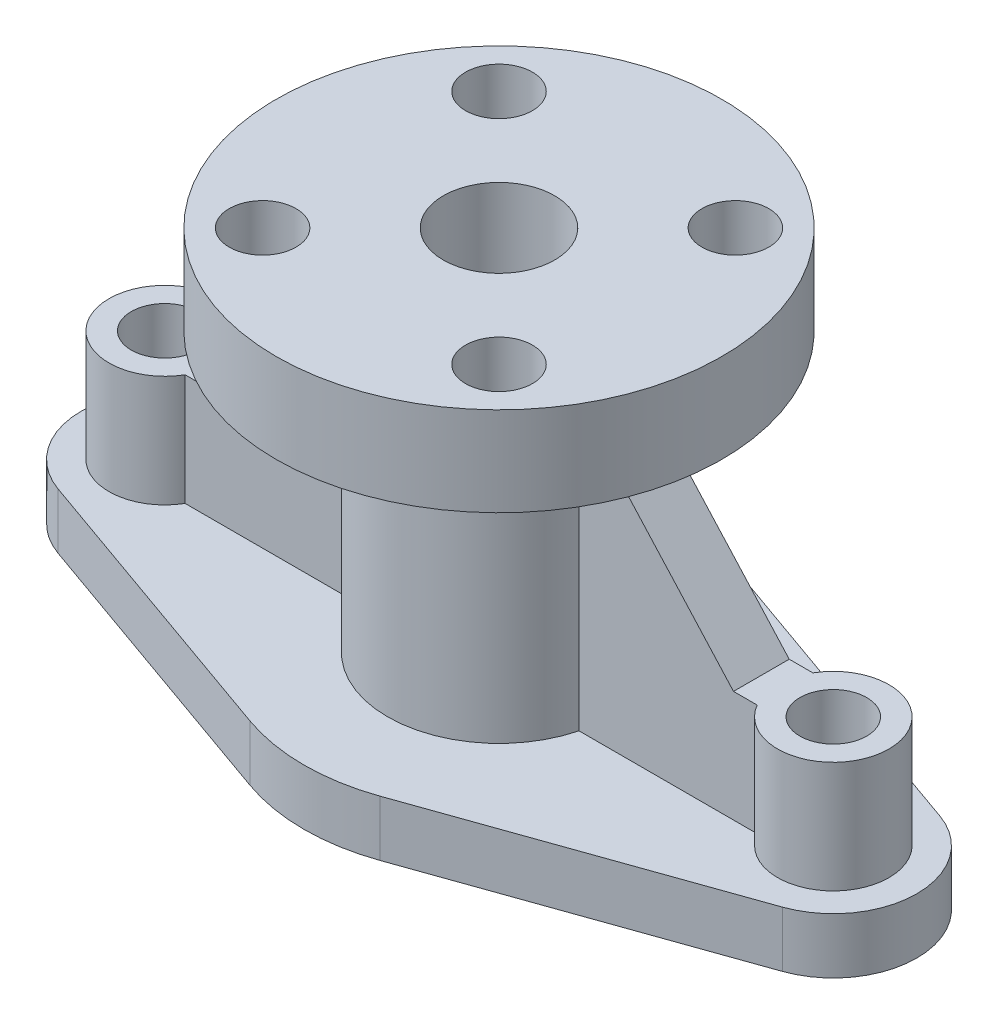
ISO-10303-21;
HEADER;
FILE_DESCRIPTION(('STEP AP214'),'2;1');
FILE_NAME('part.step','',(''),(''),'','','');
FILE_SCHEMA(('AUTOMOTIVE_DESIGN { 1 0 10303 214 1 1 1 1 }'));
ENDSEC;
DATA;
#1=APPLICATION_CONTEXT('core data for automotive mechanical design processes');
#2=APPLICATION_PROTOCOL_DEFINITION('international standard','automotive_design',2000,#1);
#3=PRODUCT_CONTEXT('',#1,'mechanical');
#4=PRODUCT('Part','Part','',(#3));
#5=PRODUCT_RELATED_PRODUCT_CATEGORY('part','',(#4));
#6=PRODUCT_DEFINITION_FORMATION('','',#4);
#7=PRODUCT_DEFINITION_CONTEXT('part definition',#1,'design');
#8=PRODUCT_DEFINITION('design','',#6,#7);
#9=PRODUCT_DEFINITION_SHAPE('','',#8);
#10=(LENGTH_UNIT() NAMED_UNIT(*) SI_UNIT(.MILLI.,.METRE.));
#11=(NAMED_UNIT(*) PLANE_ANGLE_UNIT() SI_UNIT($,.RADIAN.));
#12=(NAMED_UNIT(*) SI_UNIT($,.STERADIAN.) SOLID_ANGLE_UNIT());
#13=UNCERTAINTY_MEASURE_WITH_UNIT(LENGTH_MEASURE(1.E-05),#10,'distance_accuracy_value','');
#14=(GEOMETRIC_REPRESENTATION_CONTEXT(3) GLOBAL_UNCERTAINTY_ASSIGNED_CONTEXT((#13)) GLOBAL_UNIT_ASSIGNED_CONTEXT((#10,
#11,#12)) REPRESENTATION_CONTEXT('',''));
#15=CARTESIAN_POINT('',(0.,0.,0.));
#16=DIRECTION('',(0.,0.,1.));
#17=DIRECTION('',(1.,0.,0.));
#18=AXIS2_PLACEMENT_3D('',#15,#16,#17);
#19=CARTESIAN_POINT('',(0.,10.,0.));
#20=DIRECTION('',(0.,-1.,0.));
#21=DIRECTION('',(0.,0.,-1.));
#22=AXIS2_PLACEMENT_3D('',#19,#20,#21);
#23=CYLINDRICAL_SURFACE('',#22,5.);
#24=CARTESIAN_POINT('',(0.,0.,0.));
#25=DIRECTION('',(0.,1.,0.));
#26=DIRECTION('',(0.,0.,1.));
#27=AXIS2_PLACEMENT_3D('',#24,#25,#26);
#28=CIRCLE('',#27,5.);
#29=CARTESIAN_POINT('',(0.,0.,5.));
#30=VERTEX_POINT('',#29);
#31=EDGE_CURVE('E241',#30,#30,#28,.T.);
#32=ORIENTED_EDGE('',*,*,#31,.F.);
#33=EDGE_LOOP('',(#32));
#34=FACE_BOUND('',#33,.T.);
#35=CARTESIAN_POINT('',(0.,45.,0.));
#36=DIRECTION('',(0.,1.,0.));
#37=DIRECTION('',(0.,0.,1.));
#38=AXIS2_PLACEMENT_3D('',#35,#36,#37);
#39=CIRCLE('',#38,5.);
#40=CARTESIAN_POINT('',(0.,45.,5.));
#41=VERTEX_POINT('',#40);
#42=EDGE_CURVE('E47',#41,#41,#39,.T.);
#43=ORIENTED_EDGE('',*,*,#42,.T.);
#44=EDGE_LOOP('',(#43));
#45=FACE_BOUND('',#44,.T.);
#46=ADVANCED_FACE('F44',(#34,#45),#23,.F.);
#47=CARTESIAN_POINT('',(0.,30.,0.));
#48=DIRECTION('',(0.,-1.,0.));
#49=DIRECTION('',(0.,0.,-1.));
#50=AXIS2_PLACEMENT_3D('',#47,#48,#49);
#51=CYLINDRICAL_SURFACE('',#50,20.);
#52=DIRECTION('',(0.,-1.,0.));
#53=VECTOR('',#52,1.);
#54=CARTESIAN_POINT('',(19.3649167310371,30.,-5.));
#55=LINE('',#54,#53);
#56=CARTESIAN_POINT('',(19.3649167310371,10.,-5.));
#57=VERTEX_POINT('',#56);
#58=CARTESIAN_POINT('',(19.3649167310371,60.,-5.));
#59=VERTEX_POINT('',#58);
#60=EDGE_CURVE('E61',#57,#59,#55,.F.);
#61=ORIENTED_EDGE('',*,*,#60,.F.);
#62=CARTESIAN_POINT('',(0.,10.,0.));
#63=DIRECTION('',(0.,1.,0.));
#64=DIRECTION('',(0.,0.,1.));
#65=AXIS2_PLACEMENT_3D('',#62,#63,#64);
#66=CIRCLE('',#65,20.);
#67=CARTESIAN_POINT('',(-19.3649167310371,10.,-5.));
#68=VERTEX_POINT('',#67);
#69=EDGE_CURVE('E230',#57,#68,#66,.T.);
#70=ORIENTED_EDGE('',*,*,#69,.T.);
#71=DIRECTION('',(0.,-1.,0.));
#72=VECTOR('',#71,1.);
#73=CARTESIAN_POINT('',(-19.3649167310371,30.,-5.));
#74=LINE('',#73,#72);
#75=CARTESIAN_POINT('',(-19.3649167310371,60.,-5.));
#76=VERTEX_POINT('',#75);
#77=EDGE_CURVE('E215',#76,#68,#74,.T.);
#78=ORIENTED_EDGE('',*,*,#77,.F.);
#79=CARTESIAN_POINT('',(0.,60.,0.));
#80=DIRECTION('',(0.,1.,0.));
#81=DIRECTION('',(0.,0.,1.));
#82=AXIS2_PLACEMENT_3D('',#79,#80,#81);
#83=CIRCLE('',#82,20.);
#84=EDGE_CURVE('E202',#59,#76,#83,.T.);
#85=ORIENTED_EDGE('',*,*,#84,.F.);
#86=EDGE_LOOP('',(#61,#70,#78,#85));
#87=FACE_BOUND('',#86,.T.);
#88=ADVANCED_FACE('F346',(#87),#51,.T.);
#89=CARTESIAN_POINT('',(0.,10.,0.));
#90=DIRECTION('',(0.,1.,0.));
#91=DIRECTION('',(0.,0.,1.));
#92=AXIS2_PLACEMENT_3D('',#89,#90,#91);
#93=PLANE('',#92);
#94=DIRECTION('',(1.,0.,0.));
#95=VECTOR('',#94,1.);
#96=CARTESIAN_POINT('',(17.3522070106996,9.99999999999999,5.));
#97=LINE('',#96,#95);
#98=CARTESIAN_POINT('',(19.3649167310371,10.,5.));
#99=VERTEX_POINT('',#98);
#100=CARTESIAN_POINT('',(51.3397459621556,10.,5.));
#101=VERTEX_POINT('',#100);
#102=EDGE_CURVE('E68',#99,#101,#97,.T.);
#103=ORIENTED_EDGE('',*,*,#102,.F.);
#104=CARTESIAN_POINT('',(-19.3649167310371,10.,5.));
#105=VERTEX_POINT('',#104);
#106=EDGE_CURVE('E234',#105,#99,#66,.T.);
#107=ORIENTED_EDGE('',*,*,#106,.F.);
#108=DIRECTION('',(1.,0.,0.));
#109=VECTOR('',#108,1.);
#110=CARTESIAN_POINT('',(-52.,10.,5.));
#111=LINE('',#110,#109);
#112=CARTESIAN_POINT('',(-51.3397459621556,10.,5.));
#113=VERTEX_POINT('',#112);
#114=EDGE_CURVE('E198',#113,#105,#111,.T.);
#115=ORIENTED_EDGE('',*,*,#114,.F.);
#116=CARTESIAN_POINT('',(-60.,10.,0.));
#117=DIRECTION('',(0.,1.,0.));
#118=DIRECTION('',(0.,0.,1.));
#119=AXIS2_PLACEMENT_3D('',#116,#117,#118);
#120=CIRCLE('',#119,10.);
#121=CARTESIAN_POINT('',(-51.3397459621556,10.,-5.));
#122=VERTEX_POINT('',#121);
#123=EDGE_CURVE('E226',#122,#113,#120,.T.);
#124=ORIENTED_EDGE('',*,*,#123,.F.);
#125=DIRECTION('',(1.,0.,0.));
#126=VECTOR('',#125,1.);
#127=CARTESIAN_POINT('',(-52.,10.,-5.));
#128=LINE('',#127,#126);
#129=EDGE_CURVE('E532',#122,#68,#128,.T.);
#130=ORIENTED_EDGE('',*,*,#129,.T.);
#131=ORIENTED_EDGE('',*,*,#69,.F.);
#132=DIRECTION('',(1.,0.,0.));
#133=VECTOR('',#132,1.);
#134=CARTESIAN_POINT('',(17.3522070106996,9.99999999999999,-5.));
#135=LINE('',#134,#133);
#136=CARTESIAN_POINT('',(51.3397459621556,10.,-5.));
#137=VERTEX_POINT('',#136);
#138=EDGE_CURVE('E509',#57,#137,#135,.T.);
#139=ORIENTED_EDGE('',*,*,#138,.T.);
#140=CARTESIAN_POINT('',(60.,10.,0.));
#141=DIRECTION('',(0.,1.,0.));
#142=DIRECTION('',(0.,0.,1.));
#143=AXIS2_PLACEMENT_3D('',#140,#141,#142);
#144=CIRCLE('',#143,9.99999999999999);
#145=EDGE_CURVE('E217',#101,#137,#144,.T.);
#146=ORIENTED_EDGE('',*,*,#145,.F.);
#147=EDGE_LOOP('',(#103,#107,#115,#124,#130,#131,#139,#146));
#148=FACE_BOUND('',#147,.T.);
#149=CARTESIAN_POINT('',(0.,10.,0.));
#150=DIRECTION('',(0.,1.,0.));
#151=DIRECTION('',(0.,0.,1.));
#152=AXIS2_PLACEMENT_3D('',#149,#150,#151);
#153=CIRCLE('',#152,35.);
#154=CARTESIAN_POINT('',(11.6666666666667,10.,-32.9983164553722));
#155=VERTEX_POINT('',#154);
#156=CARTESIAN_POINT('',(-11.6666666666667,10.,-32.9983164553722));
#157=VERTEX_POINT('',#156);
#158=EDGE_CURVE('E245',#155,#157,#153,.T.);
#159=ORIENTED_EDGE('',*,*,#158,.T.);
#160=DIRECTION('',(-0.942809041582063,0.,0.333333333333334));
#161=VECTOR('',#160,1.);
#162=CARTESIAN_POINT('',(-11.6666666666667,10.,-32.9983164553722));
#163=LINE('',#162,#161);
#164=CARTESIAN_POINT('',(-65.,10.,-14.1421356237309));
#165=VERTEX_POINT('',#164);
#166=EDGE_CURVE('E249',#157,#165,#163,.T.);
#167=ORIENTED_EDGE('',*,*,#166,.T.);
#168=CARTESIAN_POINT('',(-60.,10.,0.));
#169=DIRECTION('',(0.,1.,0.));
#170=DIRECTION('',(0.,0.,1.));
#171=AXIS2_PLACEMENT_3D('',#168,#169,#170);
#172=CIRCLE('',#171,15.);
#173=CARTESIAN_POINT('',(-65.,10.,14.1421356237309));
#174=VERTEX_POINT('',#173);
#175=EDGE_CURVE('E253',#165,#174,#172,.T.);
#176=ORIENTED_EDGE('',*,*,#175,.T.);
#177=DIRECTION('',(0.942809041582063,0.,0.333333333333334));
#178=VECTOR('',#177,1.);
#179=CARTESIAN_POINT('',(-65.,10.,14.1421356237309));
#180=LINE('',#179,#178);
#181=CARTESIAN_POINT('',(-11.6666666666667,10.,32.9983164553722));
#182=VERTEX_POINT('',#181);
#183=EDGE_CURVE('E251',#174,#182,#180,.T.);
#184=ORIENTED_EDGE('',*,*,#183,.T.);
#185=CARTESIAN_POINT('',(0.,10.,0.));
#186=DIRECTION('',(0.,1.,0.));
#187=DIRECTION('',(0.,0.,1.));
#188=AXIS2_PLACEMENT_3D('',#185,#186,#187);
#189=CIRCLE('',#188,35.);
#190=CARTESIAN_POINT('',(11.6666666666667,10.,32.9983164553722));
#191=VERTEX_POINT('',#190);
#192=EDGE_CURVE('E254',#182,#191,#189,.T.);
#193=ORIENTED_EDGE('',*,*,#192,.T.);
#194=DIRECTION('',(0.942809041582063,0.,-0.333333333333334));
#195=VECTOR('',#194,1.);
#196=CARTESIAN_POINT('',(11.6666666666667,10.,32.9983164553722));
#197=LINE('',#196,#195);
#198=CARTESIAN_POINT('',(65.,10.,14.1421356237309));
#199=VERTEX_POINT('',#198);
#200=EDGE_CURVE('E260',#191,#199,#197,.T.);
#201=ORIENTED_EDGE('',*,*,#200,.T.);
#202=CARTESIAN_POINT('',(60.,10.,0.));
#203=DIRECTION('',(0.,1.,0.));
#204=DIRECTION('',(0.,0.,1.));
#205=AXIS2_PLACEMENT_3D('',#202,#203,#204);
#206=CIRCLE('',#205,15.);
#207=CARTESIAN_POINT('',(65.,10.,-14.1421356237309));
#208=VERTEX_POINT('',#207);
#209=EDGE_CURVE('E259',#199,#208,#206,.T.);
#210=ORIENTED_EDGE('',*,*,#209,.T.);
#211=DIRECTION('',(-0.942809041582063,0.,-0.333333333333334));
#212=VECTOR('',#211,1.);
#213=CARTESIAN_POINT('',(11.6666666666667,10.,-32.9983164553722));
#214=LINE('',#213,#212);
#215=EDGE_CURVE('E261',#208,#155,#214,.T.);
#216=ORIENTED_EDGE('',*,*,#215,.T.);
#217=EDGE_LOOP('',(#159,#167,#176,#184,#193,#201,#210,#216));
#218=FACE_BOUND('',#217,.T.);
#219=ADVANCED_FACE('F321',(#148,#218),#93,.T.);
#220=CARTESIAN_POINT('',(0.,0.,0.));
#221=DIRECTION('',(0.,1.,0.));
#222=DIRECTION('',(0.,0.,1.));
#223=AXIS2_PLACEMENT_3D('',#220,#221,#222);
#224=PLANE('',#223);
#225=CARTESIAN_POINT('',(0.,0.,0.));
#226=DIRECTION('',(0.,1.,0.));
#227=DIRECTION('',(0.,0.,1.));
#228=AXIS2_PLACEMENT_3D('',#225,#226,#227);
#229=CIRCLE('',#228,35.);
#230=CARTESIAN_POINT('',(11.6666666666667,0.,-32.9983164553722));
#231=VERTEX_POINT('',#230);
#232=CARTESIAN_POINT('',(-11.6666666666667,0.,-32.9983164553722));
#233=VERTEX_POINT('',#232);
#234=EDGE_CURVE('E243',#231,#233,#229,.T.);
#235=ORIENTED_EDGE('',*,*,#234,.F.);
#236=DIRECTION('',(-0.942809041582063,0.,-0.333333333333334));
#237=VECTOR('',#236,1.);
#238=CARTESIAN_POINT('',(11.6666666666667,0.,-32.9983164553722));
#239=LINE('',#238,#237);
#240=CARTESIAN_POINT('',(65.,0.,-14.1421356237309));
#241=VERTEX_POINT('',#240);
#242=EDGE_CURVE('E248',#241,#231,#239,.T.);
#243=ORIENTED_EDGE('',*,*,#242,.F.);
#244=CARTESIAN_POINT('',(60.,0.,0.));
#245=DIRECTION('',(0.,1.,0.));
#246=DIRECTION('',(0.,0.,1.));
#247=AXIS2_PLACEMENT_3D('',#244,#245,#246);
#248=CIRCLE('',#247,15.);
#249=CARTESIAN_POINT('',(65.,0.,14.1421356237309));
#250=VERTEX_POINT('',#249);
#251=EDGE_CURVE('E277',#250,#241,#248,.T.);
#252=ORIENTED_EDGE('',*,*,#251,.F.);
#253=DIRECTION('',(0.942809041582063,0.,-0.333333333333334));
#254=VECTOR('',#253,1.);
#255=CARTESIAN_POINT('',(11.6666666666667,0.,32.9983164553722));
#256=LINE('',#255,#254);
#257=CARTESIAN_POINT('',(11.6666666666667,0.,32.9983164553722));
#258=VERTEX_POINT('',#257);
#259=EDGE_CURVE('E273',#258,#250,#256,.T.);
#260=ORIENTED_EDGE('',*,*,#259,.F.);
#261=CARTESIAN_POINT('',(0.,0.,0.));
#262=DIRECTION('',(0.,1.,0.));
#263=DIRECTION('',(0.,0.,1.));
#264=AXIS2_PLACEMENT_3D('',#261,#262,#263);
#265=CIRCLE('',#264,35.);
#266=CARTESIAN_POINT('',(-11.6666666666667,0.,32.9983164553722));
#267=VERTEX_POINT('',#266);
#268=EDGE_CURVE('E275',#267,#258,#265,.T.);
#269=ORIENTED_EDGE('',*,*,#268,.F.);
#270=DIRECTION('',(0.942809041582063,0.,0.333333333333334));
#271=VECTOR('',#270,1.);
#272=CARTESIAN_POINT('',(-65.,0.,14.1421356237309));
#273=LINE('',#272,#271);
#274=CARTESIAN_POINT('',(-65.,0.,14.1421356237309));
#275=VERTEX_POINT('',#274);
#276=EDGE_CURVE('E269',#275,#267,#273,.T.);
#277=ORIENTED_EDGE('',*,*,#276,.F.);
#278=CARTESIAN_POINT('',(-60.,0.,0.));
#279=DIRECTION('',(0.,1.,0.));
#280=DIRECTION('',(0.,0.,1.));
#281=AXIS2_PLACEMENT_3D('',#278,#279,#280);
#282=CIRCLE('',#281,15.);
#283=CARTESIAN_POINT('',(-65.,0.,-14.1421356237309));
#284=VERTEX_POINT('',#283);
#285=EDGE_CURVE('E268',#284,#275,#282,.T.);
#286=ORIENTED_EDGE('',*,*,#285,.F.);
#287=DIRECTION('',(-0.942809041582063,0.,0.333333333333334));
#288=VECTOR('',#287,1.);
#289=CARTESIAN_POINT('',(-11.6666666666667,0.,-32.9983164553722));
#290=LINE('',#289,#288);
#291=EDGE_CURVE('E266',#233,#284,#290,.T.);
#292=ORIENTED_EDGE('',*,*,#291,.F.);
#293=EDGE_LOOP('',(#235,#243,#252,#260,#269,#277,#286,#292));
#294=FACE_BOUND('',#293,.T.);
#295=ORIENTED_EDGE('',*,*,#31,.T.);
#296=EDGE_LOOP('',(#295));
#297=FACE_BOUND('',#296,.T.);
#298=CARTESIAN_POINT('',(-60.,0.,0.));
#299=DIRECTION('',(0.,1.,0.));
#300=DIRECTION('',(0.,0.,1.));
#301=AXIS2_PLACEMENT_3D('',#298,#299,#300);
#302=CIRCLE('',#301,6.);
#303=CARTESIAN_POINT('',(-60.,0.,6.));
#304=VERTEX_POINT('',#303);
#305=EDGE_CURVE('E236',#304,#304,#302,.T.);
#306=ORIENTED_EDGE('',*,*,#305,.T.);
#307=EDGE_LOOP('',(#306));
#308=FACE_BOUND('',#307,.T.);
#309=CARTESIAN_POINT('',(60.,0.,0.));
#310=DIRECTION('',(0.,1.,0.));
#311=DIRECTION('',(0.,0.,1.));
#312=AXIS2_PLACEMENT_3D('',#309,#310,#311);
#313=CIRCLE('',#312,6.);
#314=CARTESIAN_POINT('',(60.,0.,6.));
#315=VERTEX_POINT('',#314);
#316=EDGE_CURVE('E235',#315,#315,#313,.T.);
#317=ORIENTED_EDGE('',*,*,#316,.T.);
#318=EDGE_LOOP('',(#317));
#319=FACE_BOUND('',#318,.T.);
#320=ADVANCED_FACE('F307',(#294,#297,#308,#319),#224,.F.);
#321=CARTESIAN_POINT('',(0.,10.,0.));
#322=DIRECTION('',(0.,-1.,0.));
#323=DIRECTION('',(0.,0.,-1.));
#324=AXIS2_PLACEMENT_3D('',#321,#322,#323);
#325=CYLINDRICAL_SURFACE('',#324,35.);
#326=ORIENTED_EDGE('',*,*,#234,.T.);
#327=DIRECTION('',(0.,-1.,0.));
#328=VECTOR('',#327,1.);
#329=CARTESIAN_POINT('',(-11.6666666666667,10.,-32.9983164553722));
#330=LINE('',#329,#328);
#331=EDGE_CURVE('E11',#157,#233,#330,.T.);
#332=ORIENTED_EDGE('',*,*,#331,.F.);
#333=ORIENTED_EDGE('',*,*,#158,.F.);
#334=DIRECTION('',(0.,-1.,0.));
#335=VECTOR('',#334,1.);
#336=CARTESIAN_POINT('',(11.6666666666667,10.,-32.9983164553722));
#337=LINE('',#336,#335);
#338=EDGE_CURVE('E263',#155,#231,#337,.T.);
#339=ORIENTED_EDGE('',*,*,#338,.T.);
#340=EDGE_LOOP('',(#326,#332,#333,#339));
#341=FACE_BOUND('',#340,.T.);
#342=ADVANCED_FACE('F50',(#341),#325,.T.);
#343=CARTESIAN_POINT('',(-11.6666666666667,10.,-32.9983164553722));
#344=DIRECTION('',(0.333333333333334,0.,0.942809041582063));
#345=DIRECTION('',(0.942809041582063,0.,-0.333333333333334));
#346=AXIS2_PLACEMENT_3D('',#343,#344,#345);
#347=PLANE('',#346);
#348=ORIENTED_EDGE('',*,*,#291,.T.);
#349=DIRECTION('',(0.,-1.,0.));
#350=VECTOR('',#349,1.);
#351=CARTESIAN_POINT('',(-65.,10.,-14.1421356237309));
#352=LINE('',#351,#350);
#353=EDGE_CURVE('E53',#165,#284,#352,.T.);
#354=ORIENTED_EDGE('',*,*,#353,.F.);
#355=ORIENTED_EDGE('',*,*,#166,.F.);
#356=ORIENTED_EDGE('',*,*,#331,.T.);
#357=EDGE_LOOP('',(#348,#354,#355,#356));
#358=FACE_BOUND('',#357,.T.);
#359=ADVANCED_FACE('F324',(#358),#347,.F.);
#360=CARTESIAN_POINT('',(-60.,10.,0.));
#361=DIRECTION('',(0.,-1.,0.));
#362=DIRECTION('',(0.,0.,-1.));
#363=AXIS2_PLACEMENT_3D('',#360,#361,#362);
#364=CYLINDRICAL_SURFACE('',#363,15.);
#365=ORIENTED_EDGE('',*,*,#285,.T.);
#366=DIRECTION('',(0.,-1.,0.));
#367=VECTOR('',#366,1.);
#368=CARTESIAN_POINT('',(-65.,10.,14.1421356237309));
#369=LINE('',#368,#367);
#370=EDGE_CURVE('E291',#174,#275,#369,.T.);
#371=ORIENTED_EDGE('',*,*,#370,.F.);
#372=ORIENTED_EDGE('',*,*,#175,.F.);
#373=ORIENTED_EDGE('',*,*,#353,.T.);
#374=EDGE_LOOP('',(#365,#371,#372,#373));
#375=FACE_BOUND('',#374,.T.);
#376=ADVANCED_FACE('F301',(#375),#364,.T.);
#377=CARTESIAN_POINT('',(-65.,10.,14.1421356237309));
#378=DIRECTION('',(0.333333333333334,0.,-0.942809041582063));
#379=DIRECTION('',(-0.942809041582063,0.,-0.333333333333334));
#380=AXIS2_PLACEMENT_3D('',#377,#378,#379);
#381=PLANE('',#380);
#382=ORIENTED_EDGE('',*,*,#276,.T.);
#383=DIRECTION('',(0.,-1.,0.));
#384=VECTOR('',#383,1.);
#385=CARTESIAN_POINT('',(-11.6666666666667,10.,32.9983164553722));
#386=LINE('',#385,#384);
#387=EDGE_CURVE('E290',#182,#267,#386,.T.);
#388=ORIENTED_EDGE('',*,*,#387,.F.);
#389=ORIENTED_EDGE('',*,*,#183,.F.);
#390=ORIENTED_EDGE('',*,*,#370,.T.);
#391=EDGE_LOOP('',(#382,#388,#389,#390));
#392=FACE_BOUND('',#391,.T.);
#393=ADVANCED_FACE('F311',(#392),#381,.F.);
#394=CARTESIAN_POINT('',(0.,10.,0.));
#395=DIRECTION('',(0.,-1.,0.));
#396=DIRECTION('',(0.,0.,-1.));
#397=AXIS2_PLACEMENT_3D('',#394,#395,#396);
#398=CYLINDRICAL_SURFACE('',#397,35.);
#399=ORIENTED_EDGE('',*,*,#268,.T.);
#400=DIRECTION('',(0.,-1.,0.));
#401=VECTOR('',#400,1.);
#402=CARTESIAN_POINT('',(11.6666666666667,10.,32.9983164553722));
#403=LINE('',#402,#401);
#404=EDGE_CURVE('E287',#191,#258,#403,.T.);
#405=ORIENTED_EDGE('',*,*,#404,.F.);
#406=ORIENTED_EDGE('',*,*,#192,.F.);
#407=ORIENTED_EDGE('',*,*,#387,.T.);
#408=EDGE_LOOP('',(#399,#405,#406,#407));
#409=FACE_BOUND('',#408,.T.);
#410=ADVANCED_FACE('F320',(#409),#398,.T.);
#411=CARTESIAN_POINT('',(11.6666666666667,10.,32.9983164553722));
#412=DIRECTION('',(-0.333333333333334,0.,-0.942809041582063));
#413=DIRECTION('',(-0.942809041582063,0.,0.333333333333334));
#414=AXIS2_PLACEMENT_3D('',#411,#412,#413);
#415=PLANE('',#414);
#416=ORIENTED_EDGE('',*,*,#259,.T.);
#417=DIRECTION('',(0.,-1.,0.));
#418=VECTOR('',#417,1.);
#419=CARTESIAN_POINT('',(65.,10.,14.1421356237309));
#420=LINE('',#419,#418);
#421=EDGE_CURVE('E283',#199,#250,#420,.T.);
#422=ORIENTED_EDGE('',*,*,#421,.F.);
#423=ORIENTED_EDGE('',*,*,#200,.F.);
#424=ORIENTED_EDGE('',*,*,#404,.T.);
#425=EDGE_LOOP('',(#416,#422,#423,#424));
#426=FACE_BOUND('',#425,.T.);
#427=ADVANCED_FACE('F339',(#426),#415,.F.);
#428=CARTESIAN_POINT('',(60.,10.,0.));
#429=DIRECTION('',(0.,-1.,0.));
#430=DIRECTION('',(0.,0.,-1.));
#431=AXIS2_PLACEMENT_3D('',#428,#429,#430);
#432=CYLINDRICAL_SURFACE('',#431,15.);
#433=ORIENTED_EDGE('',*,*,#251,.T.);
#434=DIRECTION('',(0.,-1.,0.));
#435=VECTOR('',#434,1.);
#436=CARTESIAN_POINT('',(65.,10.,-14.1421356237309));
#437=LINE('',#436,#435);
#438=EDGE_CURVE('E281',#208,#241,#437,.T.);
#439=ORIENTED_EDGE('',*,*,#438,.F.);
#440=ORIENTED_EDGE('',*,*,#209,.F.);
#441=ORIENTED_EDGE('',*,*,#421,.T.);
#442=EDGE_LOOP('',(#433,#439,#440,#441));
#443=FACE_BOUND('',#442,.T.);
#444=ADVANCED_FACE('F336',(#443),#432,.T.);
#445=CARTESIAN_POINT('',(11.6666666666667,10.,-32.9983164553722));
#446=DIRECTION('',(-0.333333333333334,0.,0.942809041582063));
#447=DIRECTION('',(0.942809041582063,0.,0.333333333333334));
#448=AXIS2_PLACEMENT_3D('',#445,#446,#447);
#449=PLANE('',#448);
#450=ORIENTED_EDGE('',*,*,#242,.T.);
#451=ORIENTED_EDGE('',*,*,#338,.F.);
#452=ORIENTED_EDGE('',*,*,#215,.F.);
#453=ORIENTED_EDGE('',*,*,#438,.T.);
#454=EDGE_LOOP('',(#450,#451,#452,#453));
#455=FACE_BOUND('',#454,.T.);
#456=ADVANCED_FACE('F332',(#455),#449,.F.);
#457=CARTESIAN_POINT('',(-60.,10.,0.));
#458=DIRECTION('',(0.,-1.,0.));
#459=DIRECTION('',(0.,0.,-1.));
#460=AXIS2_PLACEMENT_3D('',#457,#458,#459);
#461=CYLINDRICAL_SURFACE('',#460,6.);
#462=ORIENTED_EDGE('',*,*,#305,.F.);
#463=EDGE_LOOP('',(#462));
#464=FACE_BOUND('',#463,.T.);
#465=CARTESIAN_POINT('',(-60.,30.,0.));
#466=DIRECTION('',(0.,1.,0.));
#467=DIRECTION('',(0.,0.,1.));
#468=AXIS2_PLACEMENT_3D('',#465,#466,#467);
#469=CIRCLE('',#468,6.);
#470=CARTESIAN_POINT('',(-60.,30.,6.));
#471=VERTEX_POINT('',#470);
#472=EDGE_CURVE('E225',#471,#471,#469,.T.);
#473=ORIENTED_EDGE('',*,*,#472,.T.);
#474=EDGE_LOOP('',(#473));
#475=FACE_BOUND('',#474,.T.);
#476=ADVANCED_FACE('F363',(#464,#475),#461,.F.);
#477=CARTESIAN_POINT('',(60.,10.,0.));
#478=DIRECTION('',(0.,-1.,0.));
#479=DIRECTION('',(0.,0.,-1.));
#480=AXIS2_PLACEMENT_3D('',#477,#478,#479);
#481=CYLINDRICAL_SURFACE('',#480,6.);
#482=ORIENTED_EDGE('',*,*,#316,.F.);
#483=EDGE_LOOP('',(#482));
#484=FACE_BOUND('',#483,.T.);
#485=CARTESIAN_POINT('',(60.,30.,0.));
#486=DIRECTION('',(0.,1.,0.));
#487=DIRECTION('',(0.,0.,1.));
#488=AXIS2_PLACEMENT_3D('',#485,#486,#487);
#489=CIRCLE('',#488,6.);
#490=CARTESIAN_POINT('',(60.,30.,6.));
#491=VERTEX_POINT('',#490);
#492=EDGE_CURVE('E204',#491,#491,#489,.T.);
#493=ORIENTED_EDGE('',*,*,#492,.T.);
#494=EDGE_LOOP('',(#493));
#495=FACE_BOUND('',#494,.T.);
#496=ADVANCED_FACE('F375',(#484,#495),#481,.F.);
#497=ORIENTED_EDGE('',*,*,#106,.T.);
#498=DIRECTION('',(0.,-1.,0.));
#499=VECTOR('',#498,1.);
#500=CARTESIAN_POINT('',(19.3649167310371,30.,5.));
#501=LINE('',#500,#499);
#502=CARTESIAN_POINT('',(19.3649167310371,60.,5.));
#503=VERTEX_POINT('',#502);
#504=EDGE_CURVE('E205',#99,#503,#501,.F.);
#505=ORIENTED_EDGE('',*,*,#504,.T.);
#506=CARTESIAN_POINT('',(-19.3649167310371,60.,5.));
#507=VERTEX_POINT('',#506);
#508=EDGE_CURVE('E189',#507,#503,#83,.T.);
#509=ORIENTED_EDGE('',*,*,#508,.F.);
#510=DIRECTION('',(0.,-1.,0.));
#511=VECTOR('',#510,1.);
#512=CARTESIAN_POINT('',(-19.3649167310371,30.,5.));
#513=LINE('',#512,#511);
#514=EDGE_CURVE('E199',#507,#105,#513,.T.);
#515=ORIENTED_EDGE('',*,*,#514,.T.);
#516=EDGE_LOOP('',(#497,#505,#509,#515));
#517=FACE_BOUND('',#516,.T.);
#518=ADVANCED_FACE('F200',(#517),#51,.T.);
#519=CARTESIAN_POINT('',(-60.,30.,0.));
#520=DIRECTION('',(0.,1.,0.));
#521=DIRECTION('',(0.,0.,1.));
#522=AXIS2_PLACEMENT_3D('',#519,#520,#521);
#523=PLANE('',#522);
#524=CARTESIAN_POINT('',(-60.,30.,0.));
#525=DIRECTION('',(0.,1.,0.));
#526=DIRECTION('',(0.,0.,1.));
#527=AXIS2_PLACEMENT_3D('',#524,#525,#526);
#528=CIRCLE('',#527,10.);
#529=CARTESIAN_POINT('',(-51.3397459621556,30.,-5.));
#530=VERTEX_POINT('',#529);
#531=CARTESIAN_POINT('',(-51.3397459621556,30.,5.));
#532=VERTEX_POINT('',#531);
#533=EDGE_CURVE('E227',#530,#532,#528,.T.);
#534=ORIENTED_EDGE('',*,*,#533,.T.);
#535=DIRECTION('',(-1.,0.,0.));
#536=VECTOR('',#535,1.);
#537=CARTESIAN_POINT('',(-47.,30.,5.));
#538=LINE('',#537,#536);
#539=CARTESIAN_POINT('',(-47.,30.,5.));
#540=VERTEX_POINT('',#539);
#541=EDGE_CURVE('E537',#540,#532,#538,.T.);
#542=ORIENTED_EDGE('',*,*,#541,.F.);
#543=DIRECTION('',(0.,0.,-1.));
#544=VECTOR('',#543,1.);
#545=CARTESIAN_POINT('',(-47.,30.,5.));
#546=LINE('',#545,#544);
#547=CARTESIAN_POINT('',(-47.,30.,-5.));
#548=VERTEX_POINT('',#547);
#549=EDGE_CURVE('E545',#540,#548,#546,.T.);
#550=ORIENTED_EDGE('',*,*,#549,.T.);
#551=DIRECTION('',(-1.,0.,0.));
#552=VECTOR('',#551,1.);
#553=CARTESIAN_POINT('',(-47.,30.,-5.));
#554=LINE('',#553,#552);
#555=EDGE_CURVE('E536',#548,#530,#554,.T.);
#556=ORIENTED_EDGE('',*,*,#555,.T.);
#557=EDGE_LOOP('',(#534,#542,#550,#556));
#558=FACE_BOUND('',#557,.T.);
#559=ORIENTED_EDGE('',*,*,#472,.F.);
#560=EDGE_LOOP('',(#559));
#561=FACE_BOUND('',#560,.T.);
#562=ADVANCED_FACE('F385',(#558,#561),#523,.T.);
#563=CARTESIAN_POINT('',(-60.,30.,0.));
#564=DIRECTION('',(0.,-1.,0.));
#565=DIRECTION('',(0.,0.,-1.));
#566=AXIS2_PLACEMENT_3D('',#563,#564,#565);
#567=CYLINDRICAL_SURFACE('',#566,10.);
#568=ORIENTED_EDGE('',*,*,#123,.T.);
#569=DIRECTION('',(0.,-1.,0.));
#570=VECTOR('',#569,1.);
#571=CARTESIAN_POINT('',(-51.3397459621556,30.,5.));
#572=LINE('',#571,#570);
#573=EDGE_CURVE('E209',#113,#532,#572,.F.);
#574=ORIENTED_EDGE('',*,*,#573,.T.);
#575=ORIENTED_EDGE('',*,*,#533,.F.);
#576=DIRECTION('',(0.,-1.,0.));
#577=VECTOR('',#576,1.);
#578=CARTESIAN_POINT('',(-51.3397459621556,30.,-5.));
#579=LINE('',#578,#577);
#580=EDGE_CURVE('E551',#122,#530,#579,.F.);
#581=ORIENTED_EDGE('',*,*,#580,.F.);
#582=EDGE_LOOP('',(#568,#574,#575,#581));
#583=FACE_BOUND('',#582,.T.);
#584=ADVANCED_FACE('F383',(#583),#567,.T.);
#585=CARTESIAN_POINT('',(60.,30.,0.));
#586=DIRECTION('',(0.,1.,0.));
#587=DIRECTION('',(0.,0.,1.));
#588=AXIS2_PLACEMENT_3D('',#585,#586,#587);
#589=PLANE('',#588);
#590=DIRECTION('',(-1.,0.,0.));
#591=VECTOR('',#590,1.);
#592=CARTESIAN_POINT('',(52.0907779165463,30.,5.));
#593=LINE('',#592,#591);
#594=CARTESIAN_POINT('',(51.3397459621556,30.,5.));
#595=VERTEX_POINT('',#594);
#596=CARTESIAN_POINT('',(47.0907779165463,30.,5.));
#597=VERTEX_POINT('',#596);
#598=EDGE_CURVE('E505',#595,#597,#593,.T.);
#599=ORIENTED_EDGE('',*,*,#598,.F.);
#600=CARTESIAN_POINT('',(60.,30.,0.));
#601=DIRECTION('',(0.,1.,0.));
#602=DIRECTION('',(0.,0.,1.));
#603=AXIS2_PLACEMENT_3D('',#600,#601,#602);
#604=CIRCLE('',#603,9.99999999999999);
#605=CARTESIAN_POINT('',(51.3397459621556,30.,-5.));
#606=VERTEX_POINT('',#605);
#607=EDGE_CURVE('E218',#595,#606,#604,.T.);
#608=ORIENTED_EDGE('',*,*,#607,.T.);
#609=DIRECTION('',(-1.,0.,0.));
#610=VECTOR('',#609,1.);
#611=CARTESIAN_POINT('',(52.0907779165463,30.,-5.));
#612=LINE('',#611,#610);
#613=CARTESIAN_POINT('',(47.0907779165463,30.,-5.));
#614=VERTEX_POINT('',#613);
#615=EDGE_CURVE('E513',#606,#614,#612,.T.);
#616=ORIENTED_EDGE('',*,*,#615,.T.);
#617=DIRECTION('',(0.,0.,-1.));
#618=VECTOR('',#617,1.);
#619=CARTESIAN_POINT('',(47.0907779165463,30.,5.));
#620=LINE('',#619,#618);
#621=EDGE_CURVE('E525',#597,#614,#620,.T.);
#622=ORIENTED_EDGE('',*,*,#621,.F.);
#623=EDGE_LOOP('',(#599,#608,#616,#622));
#624=FACE_BOUND('',#623,.T.);
#625=ORIENTED_EDGE('',*,*,#492,.F.);
#626=EDGE_LOOP('',(#625));
#627=FACE_BOUND('',#626,.T.);
#628=ADVANCED_FACE('F388',(#624,#627),#589,.T.);
#629=CARTESIAN_POINT('',(60.,30.,0.));
#630=DIRECTION('',(0.,-1.,0.));
#631=DIRECTION('',(0.,0.,-1.));
#632=AXIS2_PLACEMENT_3D('',#629,#630,#631);
#633=CYLINDRICAL_SURFACE('',#632,9.99999999999999);
#634=ORIENTED_EDGE('',*,*,#607,.F.);
#635=DIRECTION('',(0.,-1.,0.));
#636=VECTOR('',#635,1.);
#637=CARTESIAN_POINT('',(51.3397459621556,30.,5.));
#638=LINE('',#637,#636);
#639=EDGE_CURVE('E535',#595,#101,#638,.T.);
#640=ORIENTED_EDGE('',*,*,#639,.T.);
#641=ORIENTED_EDGE('',*,*,#145,.T.);
#642=DIRECTION('',(0.,-1.,0.));
#643=VECTOR('',#642,1.);
#644=CARTESIAN_POINT('',(51.3397459621556,30.,-5.));
#645=LINE('',#644,#643);
#646=EDGE_CURVE('E526',#606,#137,#645,.T.);
#647=ORIENTED_EDGE('',*,*,#646,.F.);
#648=EDGE_LOOP('',(#634,#640,#641,#647));
#649=FACE_BOUND('',#648,.T.);
#650=ADVANCED_FACE('F395',(#649),#633,.T.);
#651=CARTESIAN_POINT('',(0.,0.,5.));
#652=DIRECTION('',(0.,0.,1.));
#653=DIRECTION('',(1.,0.,0.));
#654=AXIS2_PLACEMENT_3D('',#651,#652,#653);
#655=PLANE('',#654);
#656=ORIENTED_EDGE('',*,*,#514,.F.);
#657=DIRECTION('',(-1.,0.,0.));
#658=VECTOR('',#657,1.);
#659=CARTESIAN_POINT('',(-16.5686581072496,60.,5.));
#660=LINE('',#659,#658);
#661=CARTESIAN_POINT('',(-20.,60.,5.));
#662=VERTEX_POINT('',#661);
#663=EDGE_CURVE('E183',#507,#662,#660,.T.);
#664=ORIENTED_EDGE('',*,*,#663,.T.);
#665=DIRECTION('',(-0.66896473162245,-0.743294146247166,0.));
#666=VECTOR('',#665,1.);
#667=CARTESIAN_POINT('',(-47.,30.,5.));
#668=LINE('',#667,#666);
#669=EDGE_CURVE('E195',#662,#540,#668,.T.);
#670=ORIENTED_EDGE('',*,*,#669,.T.);
#671=ORIENTED_EDGE('',*,*,#541,.T.);
#672=ORIENTED_EDGE('',*,*,#573,.F.);
#673=ORIENTED_EDGE('',*,*,#114,.T.);
#674=EDGE_LOOP('',(#656,#664,#670,#671,#672,#673));
#675=FACE_BOUND('',#674,.T.);
#676=ADVANCED_FACE('F208',(#675),#655,.T.);
#677=CARTESIAN_POINT('',(0.,0.,-5.));
#678=DIRECTION('',(0.,0.,1.));
#679=DIRECTION('',(1.,0.,0.));
#680=AXIS2_PLACEMENT_3D('',#677,#678,#679);
#681=PLANE('',#680);
#682=DIRECTION('',(-1.,0.,0.));
#683=VECTOR('',#682,1.);
#684=CARTESIAN_POINT('',(-16.5686581072496,60.,-5.));
#685=LINE('',#684,#683);
#686=CARTESIAN_POINT('',(-20.,60.,-5.));
#687=VERTEX_POINT('',#686);
#688=EDGE_CURVE('E544',#76,#687,#685,.T.);
#689=ORIENTED_EDGE('',*,*,#688,.F.);
#690=ORIENTED_EDGE('',*,*,#77,.T.);
#691=ORIENTED_EDGE('',*,*,#129,.F.);
#692=ORIENTED_EDGE('',*,*,#580,.T.);
#693=ORIENTED_EDGE('',*,*,#555,.F.);
#694=DIRECTION('',(-0.66896473162245,-0.743294146247166,0.));
#695=VECTOR('',#694,1.);
#696=CARTESIAN_POINT('',(-47.,30.,-5.));
#697=LINE('',#696,#695);
#698=EDGE_CURVE('E550',#687,#548,#697,.T.);
#699=ORIENTED_EDGE('',*,*,#698,.F.);
#700=EDGE_LOOP('',(#689,#690,#691,#692,#693,#699));
#701=FACE_BOUND('',#700,.T.);
#702=ADVANCED_FACE('F403',(#701),#681,.F.);
#703=CARTESIAN_POINT('',(-47.,30.,5.));
#704=DIRECTION('',(0.743294146247166,-0.66896473162245,0.));
#705=DIRECTION('',(0.66896473162245,0.743294146247166,0.));
#706=AXIS2_PLACEMENT_3D('',#703,#704,#705);
#707=PLANE('',#706);
#708=ORIENTED_EDGE('',*,*,#698,.T.);
#709=ORIENTED_EDGE('',*,*,#549,.F.);
#710=ORIENTED_EDGE('',*,*,#669,.F.);
#711=DIRECTION('',(0.,0.,-1.));
#712=VECTOR('',#711,1.);
#713=CARTESIAN_POINT('',(-20.,60.,5.));
#714=LINE('',#713,#712);
#715=EDGE_CURVE('E191',#662,#687,#714,.T.);
#716=ORIENTED_EDGE('',*,*,#715,.T.);
#717=EDGE_LOOP('',(#708,#709,#710,#716));
#718=FACE_BOUND('',#717,.T.);
#719=ADVANCED_FACE('F402',(#718),#707,.F.);
#720=CARTESIAN_POINT('',(0.,0.,5.));
#721=DIRECTION('',(0.,0.,1.));
#722=DIRECTION('',(1.,0.,0.));
#723=AXIS2_PLACEMENT_3D('',#720,#721,#722);
#724=PLANE('',#723);
#725=ORIENTED_EDGE('',*,*,#504,.F.);
#726=ORIENTED_EDGE('',*,*,#102,.T.);
#727=ORIENTED_EDGE('',*,*,#639,.F.);
#728=ORIENTED_EDGE('',*,*,#598,.T.);
#729=DIRECTION('',(-0.670204558894402,0.742176427298227,0.));
#730=VECTOR('',#729,1.);
#731=CARTESIAN_POINT('',(47.0907779165463,30.,5.));
#732=LINE('',#731,#730);
#733=CARTESIAN_POINT('',(20.,60.,5.));
#734=VERTEX_POINT('',#733);
#735=EDGE_CURVE('E507',#597,#734,#732,.T.);
#736=ORIENTED_EDGE('',*,*,#735,.T.);
#737=DIRECTION('',(-1.,0.,0.));
#738=VECTOR('',#737,1.);
#739=CARTESIAN_POINT('',(20.,60.,5.));
#740=LINE('',#739,#738);
#741=EDGE_CURVE('E512',#734,#503,#740,.T.);
#742=ORIENTED_EDGE('',*,*,#741,.T.);
#743=EDGE_LOOP('',(#725,#726,#727,#728,#736,#742));
#744=FACE_BOUND('',#743,.T.);
#745=ADVANCED_FACE('F404',(#744),#724,.T.);
#746=CARTESIAN_POINT('',(0.,0.,-5.));
#747=DIRECTION('',(0.,0.,1.));
#748=DIRECTION('',(1.,0.,0.));
#749=AXIS2_PLACEMENT_3D('',#746,#747,#748);
#750=PLANE('',#749);
#751=ORIENTED_EDGE('',*,*,#138,.F.);
#752=ORIENTED_EDGE('',*,*,#60,.T.);
#753=DIRECTION('',(-1.,0.,0.));
#754=VECTOR('',#753,1.);
#755=CARTESIAN_POINT('',(20.,60.,-5.));
#756=LINE('',#755,#754);
#757=CARTESIAN_POINT('',(20.,60.,-5.));
#758=VERTEX_POINT('',#757);
#759=EDGE_CURVE('E520',#758,#59,#756,.T.);
#760=ORIENTED_EDGE('',*,*,#759,.F.);
#761=DIRECTION('',(-0.670204558894402,0.742176427298227,0.));
#762=VECTOR('',#761,1.);
#763=CARTESIAN_POINT('',(47.0907779165463,30.,-5.));
#764=LINE('',#763,#762);
#765=EDGE_CURVE('E517',#614,#758,#764,.T.);
#766=ORIENTED_EDGE('',*,*,#765,.F.);
#767=ORIENTED_EDGE('',*,*,#615,.F.);
#768=ORIENTED_EDGE('',*,*,#646,.T.);
#769=EDGE_LOOP('',(#751,#752,#760,#766,#767,#768));
#770=FACE_BOUND('',#769,.T.);
#771=ADVANCED_FACE('F418',(#770),#750,.F.);
#772=CARTESIAN_POINT('',(47.0907779165463,30.,5.));
#773=DIRECTION('',(-0.742176427298227,-0.670204558894402,0.));
#774=DIRECTION('',(0.670204558894402,-0.742176427298227,0.));
#775=AXIS2_PLACEMENT_3D('',#772,#773,#774);
#776=PLANE('',#775);
#777=ORIENTED_EDGE('',*,*,#765,.T.);
#778=DIRECTION('',(0.,0.,-1.));
#779=VECTOR('',#778,1.);
#780=CARTESIAN_POINT('',(20.,60.,5.));
#781=LINE('',#780,#779);
#782=EDGE_CURVE('E514',#734,#758,#781,.T.);
#783=ORIENTED_EDGE('',*,*,#782,.F.);
#784=ORIENTED_EDGE('',*,*,#735,.F.);
#785=ORIENTED_EDGE('',*,*,#621,.T.);
#786=EDGE_LOOP('',(#777,#783,#784,#785));
#787=FACE_BOUND('',#786,.T.);
#788=ADVANCED_FACE('F412',(#787),#776,.F.);
#789=CARTESIAN_POINT('',(0.,60.,0.));
#790=DIRECTION('',(0.,1.,0.));
#791=DIRECTION('',(0.,0.,1.));
#792=AXIS2_PLACEMENT_3D('',#789,#790,#791);
#793=CONICAL_SURFACE('',#792,10.,0.26179938779915);
#794=CARTESIAN_POINT('',(0.,45.,0.));
#795=DIRECTION('',(0.,1.,0.));
#796=DIRECTION('',(0.,0.,1.));
#797=AXIS2_PLACEMENT_3D('',#794,#795,#796);
#798=CIRCLE('',#797,5.98076211353315);
#799=CARTESIAN_POINT('',(0.,45.,5.98076211353315));
#800=VERTEX_POINT('',#799);
#801=EDGE_CURVE('E498',#800,#800,#798,.T.);
#802=ORIENTED_EDGE('',*,*,#801,.F.);
#803=EDGE_LOOP('',(#802));
#804=FACE_BOUND('',#803,.T.);
#805=CARTESIAN_POINT('',(0.,60.,0.));
#806=DIRECTION('',(0.,1.,0.));
#807=DIRECTION('',(0.,0.,1.));
#808=AXIS2_PLACEMENT_3D('',#805,#806,#807);
#809=CIRCLE('',#808,10.);
#810=CARTESIAN_POINT('',(0.,60.,10.));
#811=VERTEX_POINT('',#810);
#812=EDGE_CURVE('E488',#811,#811,#809,.T.);
#813=ORIENTED_EDGE('',*,*,#812,.T.);
#814=EDGE_LOOP('',(#813));
#815=FACE_BOUND('',#814,.T.);
#816=ADVANCED_FACE('F415',(#804,#815),#793,.F.);
#817=CARTESIAN_POINT('',(0.,45.,0.));
#818=DIRECTION('',(0.,1.,0.));
#819=DIRECTION('',(0.,0.,1.));
#820=AXIS2_PLACEMENT_3D('',#817,#818,#819);
#821=PLANE('',#820);
#822=ORIENTED_EDGE('',*,*,#42,.F.);
#823=EDGE_LOOP('',(#822));
#824=FACE_BOUND('',#823,.T.);
#825=ORIENTED_EDGE('',*,*,#801,.T.);
#826=EDGE_LOOP('',(#825));
#827=FACE_BOUND('',#826,.T.);
#828=ADVANCED_FACE('F422',(#824,#827),#821,.T.);
#829=CARTESIAN_POINT('',(0.,60.,0.));
#830=DIRECTION('',(0.,1.,0.));
#831=DIRECTION('',(0.,0.,1.));
#832=AXIS2_PLACEMENT_3D('',#829,#830,#831);
#833=PLANE('',#832);
#834=CARTESIAN_POINT('',(-21.2132034355965,60.,-21.2132034355952));
#835=DIRECTION('',(0.,1.,0.));
#836=DIRECTION('',(0.,0.,1.));
#837=AXIS2_PLACEMENT_3D('',#834,#835,#836);
#838=CIRCLE('',#837,6.00000000000127);
#839=CARTESIAN_POINT('',(-21.2132034355965,60.,-15.2132034355939));
#840=VERTEX_POINT('',#839);
#841=EDGE_CURVE('E469',#840,#840,#838,.T.);
#842=ORIENTED_EDGE('',*,*,#841,.T.);
#843=EDGE_LOOP('',(#842));
#844=FACE_BOUND('',#843,.T.);
#845=CARTESIAN_POINT('',(-21.2132034355952,60.,21.2132034355976));
#846=DIRECTION('',(0.,1.,0.));
#847=DIRECTION('',(0.,0.,1.));
#848=AXIS2_PLACEMENT_3D('',#845,#846,#847);
#849=CIRCLE('',#848,6.00000000000088);
#850=CARTESIAN_POINT('',(-21.2132034355952,60.,27.2132034355985));
#851=VERTEX_POINT('',#850);
#852=EDGE_CURVE('E470',#851,#851,#849,.T.);
#853=ORIENTED_EDGE('',*,*,#852,.T.);
#854=EDGE_LOOP('',(#853));
#855=FACE_BOUND('',#854,.T.);
#856=CARTESIAN_POINT('',(21.2132034355976,60.,21.2132034355964));
#857=DIRECTION('',(0.,1.,0.));
#858=DIRECTION('',(0.,0.,1.));
#859=AXIS2_PLACEMENT_3D('',#856,#857,#858);
#860=CIRCLE('',#859,5.9999999999997);
#861=CARTESIAN_POINT('',(21.2132034355976,60.,27.2132034355961));
#862=VERTEX_POINT('',#861);
#863=EDGE_CURVE('E478',#862,#862,#860,.T.);
#864=ORIENTED_EDGE('',*,*,#863,.T.);
#865=EDGE_LOOP('',(#864));
#866=FACE_BOUND('',#865,.T.);
#867=CARTESIAN_POINT('',(21.2132034355964,60.,-21.2132034355965));
#868=DIRECTION('',(0.,1.,0.));
#869=DIRECTION('',(0.,0.,1.));
#870=AXIS2_PLACEMENT_3D('',#867,#868,#869);
#871=CIRCLE('',#870,6.);
#872=CARTESIAN_POINT('',(21.2132034355964,60.,-15.2132034355965));
#873=VERTEX_POINT('',#872);
#874=EDGE_CURVE('E485',#873,#873,#871,.T.);
#875=ORIENTED_EDGE('',*,*,#874,.T.);
#876=EDGE_LOOP('',(#875));
#877=FACE_BOUND('',#876,.T.);
#878=CARTESIAN_POINT('',(0.,60.,0.));
#879=DIRECTION('',(0.,1.,0.));
#880=DIRECTION('',(0.,0.,1.));
#881=AXIS2_PLACEMENT_3D('',#878,#879,#880);
#882=CIRCLE('',#881,40.);
#883=CARTESIAN_POINT('',(0.,60.,40.));
#884=VERTEX_POINT('',#883);
#885=EDGE_CURVE('E493',#884,#884,#882,.T.);
#886=ORIENTED_EDGE('',*,*,#885,.F.);
#887=EDGE_LOOP('',(#886));
#888=FACE_BOUND('',#887,.T.);
#889=ORIENTED_EDGE('',*,*,#663,.F.);
#890=ORIENTED_EDGE('',*,*,#508,.T.);
#891=ORIENTED_EDGE('',*,*,#741,.F.);
#892=ORIENTED_EDGE('',*,*,#782,.T.);
#893=ORIENTED_EDGE('',*,*,#759,.T.);
#894=ORIENTED_EDGE('',*,*,#84,.T.);
#895=ORIENTED_EDGE('',*,*,#688,.T.);
#896=ORIENTED_EDGE('',*,*,#715,.F.);
#897=EDGE_LOOP('',(#889,#890,#891,#892,#893,#894,#895,#896));
#898=FACE_BOUND('',#897,.T.);
#899=ADVANCED_FACE('F187',(#844,#855,#866,#877,#888,#898),#833,.F.);
#900=CARTESIAN_POINT('',(0.,76.,0.));
#901=DIRECTION('',(0.,1.,0.));
#902=DIRECTION('',(0.,0.,1.));
#903=AXIS2_PLACEMENT_3D('',#900,#901,#902);
#904=PLANE('',#903);
#905=CARTESIAN_POINT('',(-21.2132034355952,76.,21.2132034355976));
#906=DIRECTION('',(0.,1.,0.));
#907=DIRECTION('',(0.,0.,1.));
#908=AXIS2_PLACEMENT_3D('',#905,#906,#907);
#909=CIRCLE('',#908,6.00000000000088);
#910=CARTESIAN_POINT('',(-21.2132034355952,76.,27.2132034355985));
#911=VERTEX_POINT('',#910);
#912=EDGE_CURVE('E471',#911,#911,#909,.T.);
#913=ORIENTED_EDGE('',*,*,#912,.F.);
#914=EDGE_LOOP('',(#913));
#915=FACE_BOUND('',#914,.T.);
#916=CARTESIAN_POINT('',(21.2132034355964,76.,-21.2132034355965));
#917=DIRECTION('',(0.,1.,0.));
#918=DIRECTION('',(0.,0.,1.));
#919=AXIS2_PLACEMENT_3D('',#916,#917,#918);
#920=CIRCLE('',#919,6.);
#921=CARTESIAN_POINT('',(21.2132034355964,76.,-15.2132034355965));
#922=VERTEX_POINT('',#921);
#923=EDGE_CURVE('E484',#922,#922,#920,.T.);
#924=ORIENTED_EDGE('',*,*,#923,.F.);
#925=EDGE_LOOP('',(#924));
#926=FACE_BOUND('',#925,.T.);
#927=CARTESIAN_POINT('',(0.,76.,0.));
#928=DIRECTION('',(0.,1.,0.));
#929=DIRECTION('',(0.,0.,1.));
#930=AXIS2_PLACEMENT_3D('',#927,#928,#929);
#931=CIRCLE('',#930,40.);
#932=CARTESIAN_POINT('',(0.,76.,40.));
#933=VERTEX_POINT('',#932);
#934=EDGE_CURVE('E500',#933,#933,#931,.T.);
#935=ORIENTED_EDGE('',*,*,#934,.T.);
#936=EDGE_LOOP('',(#935));
#937=FACE_BOUND('',#936,.T.);
#938=CARTESIAN_POINT('',(0.,76.,0.));
#939=DIRECTION('',(0.,1.,0.));
#940=DIRECTION('',(0.,0.,1.));
#941=AXIS2_PLACEMENT_3D('',#938,#939,#940);
#942=CIRCLE('',#941,10.);
#943=CARTESIAN_POINT('',(0.,76.,10.));
#944=VERTEX_POINT('',#943);
#945=EDGE_CURVE('E491',#944,#944,#942,.T.);
#946=ORIENTED_EDGE('',*,*,#945,.F.);
#947=EDGE_LOOP('',(#946));
#948=FACE_BOUND('',#947,.T.);
#949=CARTESIAN_POINT('',(21.2132034355976,76.,21.2132034355964));
#950=DIRECTION('',(0.,1.,0.));
#951=DIRECTION('',(0.,0.,1.));
#952=AXIS2_PLACEMENT_3D('',#949,#950,#951);
#953=CIRCLE('',#952,5.9999999999997);
#954=CARTESIAN_POINT('',(21.2132034355976,76.,27.2132034355961));
#955=VERTEX_POINT('',#954);
#956=EDGE_CURVE('E479',#955,#955,#953,.T.);
#957=ORIENTED_EDGE('',*,*,#956,.F.);
#958=EDGE_LOOP('',(#957));
#959=FACE_BOUND('',#958,.T.);
#960=CARTESIAN_POINT('',(-21.2132034355965,76.,-21.2132034355952));
#961=DIRECTION('',(0.,1.,0.));
#962=DIRECTION('',(0.,0.,1.));
#963=AXIS2_PLACEMENT_3D('',#960,#961,#962);
#964=CIRCLE('',#963,6.00000000000127);
#965=CARTESIAN_POINT('',(-21.2132034355965,76.,-15.2132034355939));
#966=VERTEX_POINT('',#965);
#967=EDGE_CURVE('E465',#966,#966,#964,.T.);
#968=ORIENTED_EDGE('',*,*,#967,.F.);
#969=EDGE_LOOP('',(#968));
#970=FACE_BOUND('',#969,.T.);
#971=ADVANCED_FACE('F432',(#915,#926,#937,#948,#959,#970),#904,.T.);
#972=CARTESIAN_POINT('',(0.,76.,0.));
#973=DIRECTION('',(0.,-1.,0.));
#974=DIRECTION('',(0.,0.,-1.));
#975=AXIS2_PLACEMENT_3D('',#972,#973,#974);
#976=CYLINDRICAL_SURFACE('',#975,40.);
#977=ORIENTED_EDGE('',*,*,#934,.F.);
#978=EDGE_LOOP('',(#977));
#979=FACE_BOUND('',#978,.T.);
#980=ORIENTED_EDGE('',*,*,#885,.T.);
#981=EDGE_LOOP('',(#980));
#982=FACE_BOUND('',#981,.T.);
#983=ADVANCED_FACE('F429',(#979,#982),#976,.T.);
#984=CARTESIAN_POINT('',(0.,76.,0.));
#985=DIRECTION('',(0.,-1.,0.));
#986=DIRECTION('',(0.,0.,-1.));
#987=AXIS2_PLACEMENT_3D('',#984,#985,#986);
#988=CYLINDRICAL_SURFACE('',#987,10.);
#989=ORIENTED_EDGE('',*,*,#945,.T.);
#990=EDGE_LOOP('',(#989));
#991=FACE_BOUND('',#990,.T.);
#992=ORIENTED_EDGE('',*,*,#812,.F.);
#993=EDGE_LOOP('',(#992));
#994=FACE_BOUND('',#993,.T.);
#995=ADVANCED_FACE('F433',(#991,#994),#988,.F.);
#996=CARTESIAN_POINT('',(21.2132034355964,76.,-21.2132034355965));
#997=DIRECTION('',(0.,-1.,0.));
#998=DIRECTION('',(0.,0.,-1.));
#999=AXIS2_PLACEMENT_3D('',#996,#997,#998);
#1000=CYLINDRICAL_SURFACE('',#999,6.);
#1001=ORIENTED_EDGE('',*,*,#923,.T.);
#1002=EDGE_LOOP('',(#1001));
#1003=FACE_BOUND('',#1002,.T.);
#1004=ORIENTED_EDGE('',*,*,#874,.F.);
#1005=EDGE_LOOP('',(#1004));
#1006=FACE_BOUND('',#1005,.T.);
#1007=ADVANCED_FACE('F441',(#1003,#1006),#1000,.F.);
#1008=CARTESIAN_POINT('',(21.2132034355976,76.,21.2132034355964));
#1009=DIRECTION('',(0.,-1.,0.));
#1010=DIRECTION('',(0.,0.,-1.));
#1011=AXIS2_PLACEMENT_3D('',#1008,#1009,#1010);
#1012=CYLINDRICAL_SURFACE('',#1011,5.9999999999997);
#1013=ORIENTED_EDGE('',*,*,#956,.T.);
#1014=EDGE_LOOP('',(#1013));
#1015=FACE_BOUND('',#1014,.T.);
#1016=ORIENTED_EDGE('',*,*,#863,.F.);
#1017=EDGE_LOOP('',(#1016));
#1018=FACE_BOUND('',#1017,.T.);
#1019=ADVANCED_FACE('F449',(#1015,#1018),#1012,.F.);
#1020=CARTESIAN_POINT('',(-21.2132034355952,76.,21.2132034355976));
#1021=DIRECTION('',(0.,-1.,0.));
#1022=DIRECTION('',(0.,0.,-1.));
#1023=AXIS2_PLACEMENT_3D('',#1020,#1021,#1022);
#1024=CYLINDRICAL_SURFACE('',#1023,6.00000000000088);
#1025=ORIENTED_EDGE('',*,*,#912,.T.);
#1026=EDGE_LOOP('',(#1025));
#1027=FACE_BOUND('',#1026,.T.);
#1028=ORIENTED_EDGE('',*,*,#852,.F.);
#1029=EDGE_LOOP('',(#1028));
#1030=FACE_BOUND('',#1029,.T.);
#1031=ADVANCED_FACE('F452',(#1027,#1030),#1024,.F.);
#1032=CARTESIAN_POINT('',(-21.2132034355965,76.,-21.2132034355952));
#1033=DIRECTION('',(0.,-1.,0.));
#1034=DIRECTION('',(0.,0.,-1.));
#1035=AXIS2_PLACEMENT_3D('',#1032,#1033,#1034);
#1036=CYLINDRICAL_SURFACE('',#1035,6.00000000000127);
#1037=ORIENTED_EDGE('',*,*,#967,.T.);
#1038=EDGE_LOOP('',(#1037));
#1039=FACE_BOUND('',#1038,.T.);
#1040=ORIENTED_EDGE('',*,*,#841,.F.);
#1041=EDGE_LOOP('',(#1040));
#1042=FACE_BOUND('',#1041,.T.);
#1043=ADVANCED_FACE('F457',(#1039,#1042),#1036,.F.);
#1044=CLOSED_SHELL('',(#46,#88,#219,#320,#342,#359,#376,#393,#410,#427,#444,#456,#476,#496,#518,
#562,#584,#628,#650,#676,#702,#719,#745,#771,#788,#816,#828,#899,#971,#983,#995,#1007,#1019,
#1031,#1043));
#1045=MANIFOLD_SOLID_BREP('B2',#1044);
#1046=ADVANCED_BREP_SHAPE_REPRESENTATION('',(#18,#1045),#14);
#1047=SHAPE_DEFINITION_REPRESENTATION(#9,#1046);
ENDSEC;
END-ISO-10303-21;
